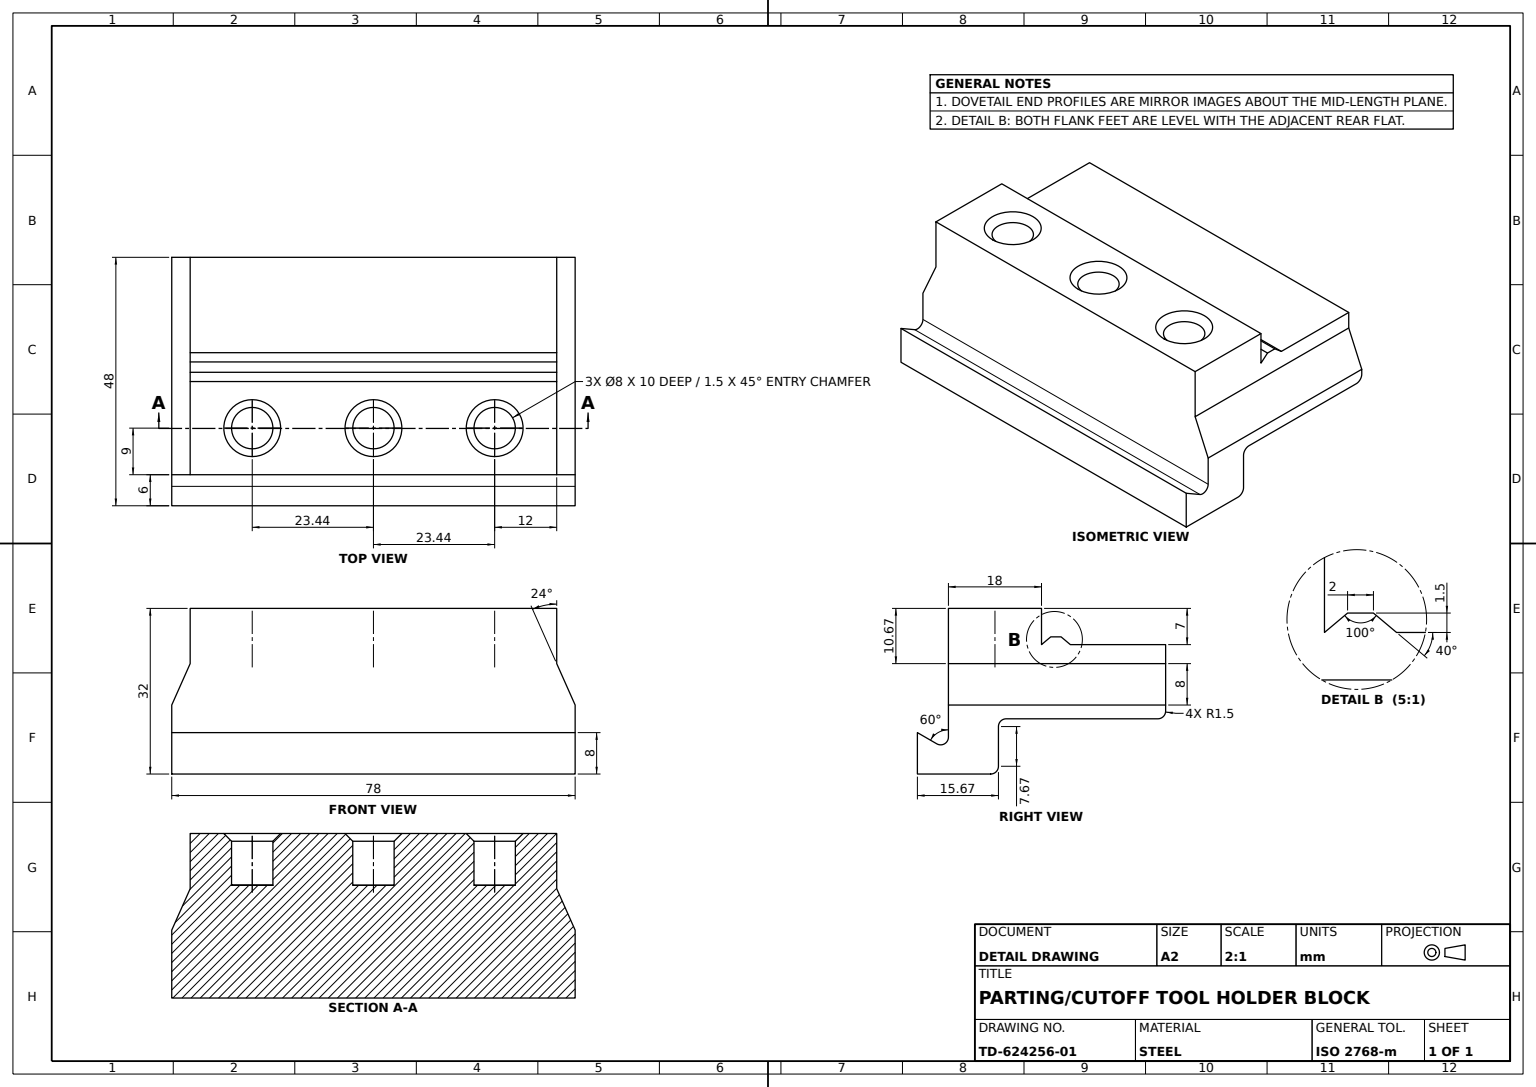
from build123d import *

# Parameters (mm, degrees)
DOVETAIL_BODY_DEPTH       = 48
GROOVE_CUT_DEPTH          = 88
MOUNTING_HOLES_LAYOUT_R   = 4
MOUNTING_HOLES_3X_8_DEPTH = 10
HOLE_CHAMFERS_1_5X45_SIZE = 1.5


with BuildPart() as part:
    # Dovetail Body Profile → Dovetail Body (new body)
    with BuildSketch(Plane.XY):
        Polygon((0, 0), (0, 13.33), (3.561829482, 21.33), (3.561829482, 32), (74.438170518, 32), (74.438170518, 21.33), (78, 13.33), (78, 0), align=None)
    extrude(amount=-DOVETAIL_BODY_DEPTH)

    # Groove Profile → Groove Cut (cut)
    with BuildSketch(Plane(origin=(78, 0, 0), x_dir=(0, 0, -1), z_dir=(1, 0, 0))):
        with BuildLine():
            Line((0, 8), (3.75, 5.834936491))
            ThreePointArc((3.75, 5.834936491), (5.25, 5.834936491), (6, 7.133974596))
            Line((6, 7.133974596), (6, 32))
            Line((6, 32), (0, 32))
            Line((0, 32), (0, 8))
        make_face()
        Polygon((48, 25), (48, 32), (24, 32), (24, 25), (25.787630389, 26.5), (27.787630389, 26.5), (29.575260778, 25), align=None)
        with BuildLine():
            Line((46.5, 10.67), (17.171381992, 10.67))
            ThreePointArc((17.171381992, 10.67), (16.11072182, 10.230660172), (15.671381992, 9.17))
            Line((15.671381992, 9.17), (15.671381992, 1.5))
            ThreePointArc((15.671381992, 1.5), (15.232042164, 0.439339828), (14.171381992, 0))
            Line((14.171381992, 0), (48, 0))
            Line((48, 0), (48, 12.17))
            ThreePointArc((48, 12.17), (47.560660172, 11.109339828), (46.5, 10.67))
        make_face()
    extrude(amount=-GROOVE_CUT_DEPTH, mode=Mode.SUBTRACT)

    # Mounting Holes Layout → Mounting Holes 3xØ8 (cut)
    with BuildSketch(Plane(origin=(0, 32, 0), x_dir=(1, 0, 0), z_dir=(0, 1, 0))):
        with Locations(Location((62.438170518, 15, 0), (0, 0, 270))):
            Circle(MOUNTING_HOLES_LAYOUT_R)
        with Locations(Location((39, 15, 0), (0, 0, 270))):
            Circle(MOUNTING_HOLES_LAYOUT_R)
        with Locations(Location((15.561829482, 15, 0), (0, 0, 270))):
            Circle(MOUNTING_HOLES_LAYOUT_R)
    extrude(amount=-MOUNTING_HOLES_3X_8_DEPTH, mode=Mode.SUBTRACT)

    # Hole Chamfers 1.5x45
    hole_chamfers_1_5x45_edges = [part.edges().sort_by_distance(p)[0] for p in [
        (62.438170518, 32, -19),
        (39, 32, -19),
        (15.561829482, 32, -19),
    ]]
    chamfer(hole_chamfers_1_5x45_edges, length=HOLE_CHAMFERS_1_5X45_SIZE)


solid = part.part
